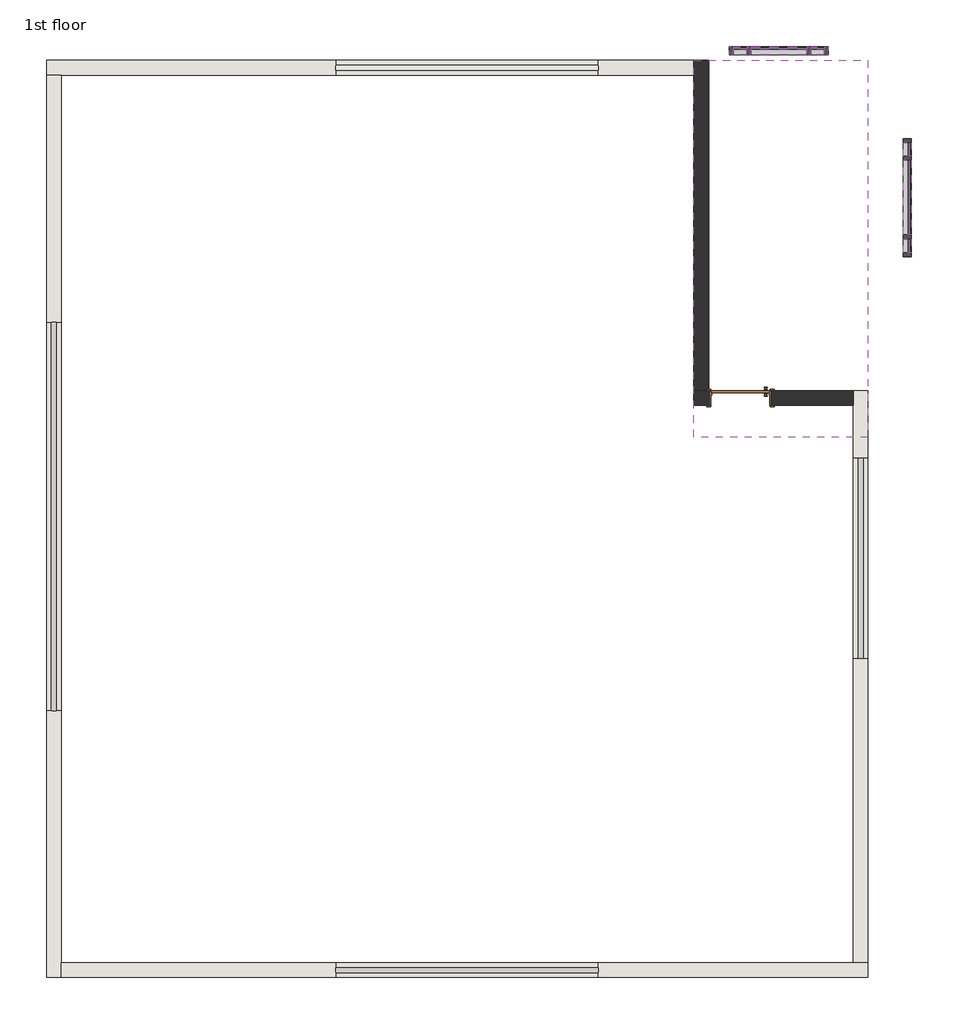
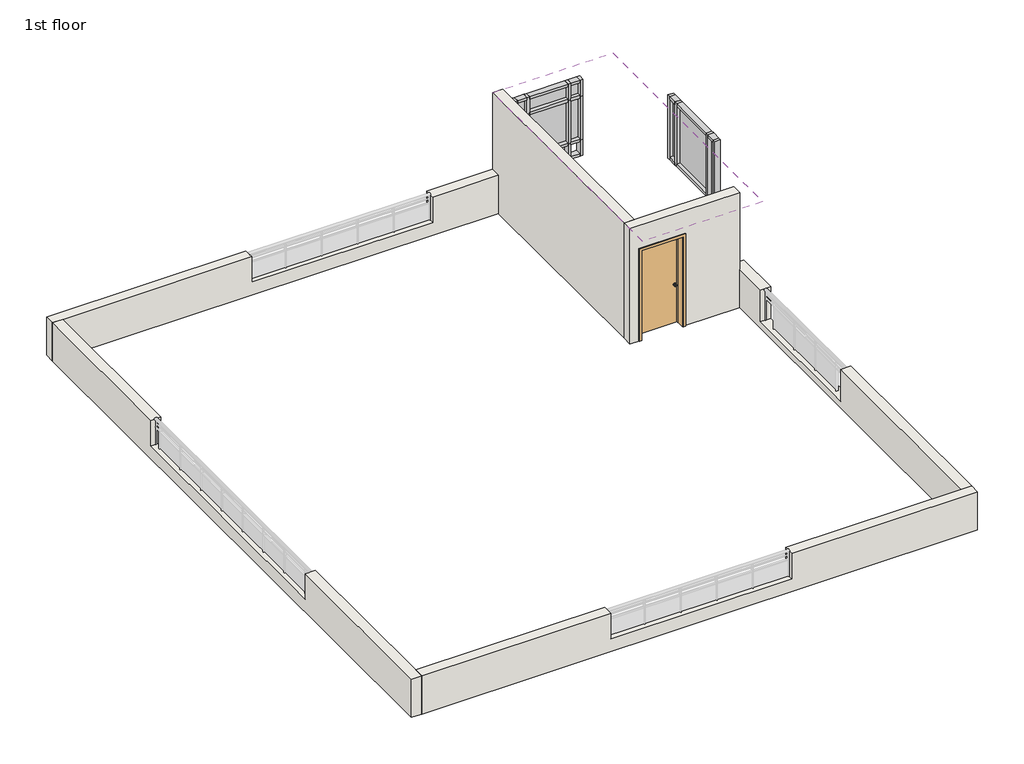
# One storey, part 1 of 2: 34 members, 9 plates, 6 walls, 1 door, 1 roof.
"""IFC4 building model written with IfcOpenShell, lengths in millimetres."""

from ifc_helpers import new_model, si_unit, frame, origin, place, context, project, spatial, polyline, outline, extrude, faceted_brep, transform, mapped, element, save
from components import door_b48525d3, member_420b45ef, member_90125dd4, member_1b4b4554, member_6b401d40, member_d98df40f, member_dfe75557, member_a5966c2a, member_b00ab025, member_467e6651, member_96c05505, member_8d8fe108, member_03a502dc, member_c5c38a7a, system_panel_glazed_475412f8, system_panel_glazed_19ddc366, system_panel_glazed_1899ac7a, system_panel_glazed_058753b2, system_panel_glazed_ee4e9f01, system_panel_glazed_f68cf4a2

model = new_model("IFC4")

# Units and contexts
model_context = context("Model", 3, world=origin())
ifc_project = project(units=[si_unit("LENGTHUNIT", "METRE", prefix="MILLI")], contexts=[model_context])

# Site, building, storey
site = spatial("IfcSite", under=ifc_project)
building = spatial("IfcBuilding", under=site)
storey = spatial("IfcBuildingStorey", under=building, Name="1st floor", Elevation=3200.4)

# Door
placement = place(None, origin())
door_shape = door_b48525d3(model_context)
element("IfcDoor", 1, ObjectType="Door-Interior-Single-Flush_Panel-Wood : 36\" x 84\"", at=placement, inside=storey, context=model_context, shape_type="MappedRepresentation", body=[
    mapped(door_shape, transform((-1718.0277598, 6738.9092801, 3200.4), x_axis=(-1.0, 0.0, 0.0), y_axis=(0.0, -1.0, 0.0), z_axis=(0.0, 0.0, 1.0))),
])

# Members
member_shape = member_420b45ef(model_context)
element("IfcMember", 2, ObjectType="Rectangular Mullion : 2.5\" x 5\" rectangular", at=placement, inside=storey, context=model_context, shape_type="MappedRepresentation", body=[
    mapped(member_shape, transform((872.7722402, 10703.2142801, 5486.4), x_axis=(0.0, 0.0, 1.0), y_axis=(1.0, 0.0, 0.0), z_axis=(0.0, 1.0, 0.0))),
])
element("IfcMember", 3, ObjectType="Rectangular Mullion : 2.5\" x 5\" rectangular", at=placement, inside=storey, context=model_context, shape_type="MappedRepresentation", body=[
    mapped(member_shape, transform((872.7722402, 9205.8842801, 5486.4), x_axis=(0.0, 0.0, 1.0), y_axis=(1.0, 0.0, 0.0), z_axis=(0.0, 1.0, 0.0))),
])
element("IfcMember", 4, ObjectType="Rectangular Mullion : 2.5\" x 5\" rectangular", at=placement, inside=storey, context=model_context, shape_type="MappedRepresentation", body=[
    mapped(member_shape, transform((-1828.7123825, 12133.2342801, 5481.32), x_axis=(0.0, 0.0, 1.0), y_axis=(0.0, 1.0, 0.0), z_axis=(-1.0, 0.0, 0.0))),
])
element("IfcMember", 5, ObjectType="Rectangular Mullion : 2.5\" x 5\" rectangular", at=placement, inside=storey, context=model_context, shape_type="MappedRepresentation", body=[
    mapped(member_shape, transform((-627.5183629, 12133.2342801, 5481.32), x_axis=(0.0, 0.0, 1.0), y_axis=(0.0, 1.0, 0.0), z_axis=(-1.0, 0.0, 0.0))),
])
member_2_shape = member_90125dd4(model_context)
element("IfcMember", 6, ObjectType="Rectangular Mullion : 2.5\" x 5\" rectangular", at=placement, inside=storey, context=model_context, shape_type="MappedRepresentation", body=[
    mapped(member_2_shape, transform((872.7722402, 8932.8342801, 5486.4), x_axis=(0.0, -1.0, 0.0), y_axis=(1.0, 0.0, 0.0), z_axis=(0.0, 0.0, 1.0))),
])
element("IfcMember", 7, ObjectType="Rectangular Mullion : 2.5\" x 5\" rectangular", at=placement, inside=storey, context=model_context, shape_type="MappedRepresentation", body=[
    mapped(member_shape, transform((872.7722402, 8996.3342801, 3976.7979445), x_axis=(0.0, 0.0, -1.0), y_axis=(1.0, 0.0, 0.0), z_axis=(0.0, -1.0, 0.0))),
])
element("IfcMember", 8, ObjectType="Rectangular Mullion : 2.5\" x 5\" rectangular", at=placement, inside=storey, context=model_context, shape_type="MappedRepresentation", body=[
    mapped(member_shape, transform((872.7722402, 10493.6642801, 3976.7979445), x_axis=(0.0, 0.0, -1.0), y_axis=(1.0, 0.0, 0.0), z_axis=(0.0, -1.0, 0.0))),
])
element("IfcMember", 9, ObjectType="Rectangular Mullion : 2.5\" x 5\" rectangular", at=placement, inside=storey, context=model_context, shape_type="MappedRepresentation", body=[
    mapped(member_shape, transform((-417.9683629, 12133.2342801, 3662.68), x_axis=(0.0, 0.0, -1.0), y_axis=(0.0, 1.0, 0.0), z_axis=(1.0, 0.0, 0.0))),
])
element("IfcMember", 10, ObjectType="Rectangular Mullion : 2.5\" x 5\" rectangular", at=placement, inside=storey, context=model_context, shape_type="MappedRepresentation", body=[
    mapped(member_shape, transform((-1619.1623825, 12133.2342801, 3662.68), x_axis=(0.0, 0.0, -1.0), y_axis=(0.0, 1.0, 0.0), z_axis=(1.0, 0.0, 0.0))),
])
element("IfcMember", 11, ObjectType="Rectangular Mullion : 2.5\" x 5\" rectangular", at=placement, inside=storey, context=model_context, shape_type="MappedRepresentation", body=[
    mapped(member_2_shape, transform((872.7722402, 10766.7142801, 3976.7979445), x_axis=(0.0, 1.0, 0.0), y_axis=(1.0, 0.0, 0.0), z_axis=(0.0, 0.0, -1.0))),
])
member_3_shape = member_1b4b4554(model_context)
element("IfcMember", 12, ObjectType="Rectangular Mullion : 2.5\" x 5\" rectangular", at=placement, inside=storey, context=model_context, shape_type="MappedRepresentation", body=[
    mapped(member_3_shape, transform((872.7722402, 9237.6342801, 5486.4), x_axis=(0.0, -1.0, 0.0), y_axis=(1.0, 0.0, 0.0), z_axis=(0.0, 0.0, 1.0))),
])
element("IfcMember", 13, ObjectType="Rectangular Mullion : 2.5\" x 5\" rectangular", at=placement, inside=storey, context=model_context, shape_type="MappedRepresentation", body=[
    mapped(member_3_shape, transform((872.7722402, 10461.9142801, 5486.4), x_axis=(0.0, -1.0, 0.0), y_axis=(1.0, 0.0, 0.0), z_axis=(0.0, 0.0, 1.0))),
])
member_4_shape = member_6b401d40(model_context)
element("IfcMember", 14, ObjectType="Rectangular Mullion : 2.5\" x 5\" rectangular", at=placement, inside=storey, context=model_context, shape_type="MappedRepresentation", body=[
    mapped(member_4_shape, transform((872.7722402, 10430.1642801, 5486.4), x_axis=(0.0, 0.0, 1.0), y_axis=(1.0, 0.0, 0.0), z_axis=(0.0, 1.0, 0.0))),
])
element("IfcMember", 15, ObjectType="Rectangular Mullion : 2.5\" x 5\" rectangular", at=placement, inside=storey, context=model_context, shape_type="MappedRepresentation", body=[
    mapped(member_4_shape, transform((872.7722402, 9269.3842801, 3976.7979445), x_axis=(0.0, 0.0, -1.0), y_axis=(1.0, 0.0, 0.0), z_axis=(0.0, -1.0, 0.0))),
])
member_5_shape = member_d98df40f(model_context)
element("IfcMember", 16, ObjectType="Rectangular Mullion : 2.5\" x 5\" rectangular", at=placement, inside=storey, context=model_context, shape_type="MappedRepresentation", body=[
    mapped(member_5_shape, transform((-354.4683629, 12133.2342801, 5481.32), x_axis=(1.0, 0.0, 0.0), y_axis=(0.0, 1.0, 0.0), z_axis=(0.0, 0.0, 1.0))),
])
member_6_shape = member_dfe75557(model_context)
element("IfcMember", 17, ObjectType="Rectangular Mullion : 2.5\" x 5\" rectangular", at=placement, inside=storey, context=model_context, shape_type="MappedRepresentation", body=[
    mapped(member_6_shape, transform((-1892.2123825, 12133.2342801, 3662.68), x_axis=(-1.0, 0.0, 0.0), y_axis=(0.0, 1.0, 0.0), z_axis=(0.0, 0.0, -1.0))),
])
member_7_shape = member_a5966c2a(model_context)
element("IfcMember", 18, ObjectType="Rectangular Mullion : 2.5\" x 5\" rectangular", at=placement, inside=storey, context=model_context, shape_type="MappedRepresentation", body=[
    mapped(member_7_shape, transform((-1828.7123825, 12133.2342801, 4043.68), x_axis=(0.0, 0.0, 1.0), y_axis=(0.0, 1.0, 0.0), z_axis=(-1.0, 0.0, 0.0))),
])
element("IfcMember", 19, ObjectType="Rectangular Mullion : 2.5\" x 5\" rectangular", at=placement, inside=storey, context=model_context, shape_type="MappedRepresentation", body=[
    mapped(member_7_shape, transform((-627.5183629, 12133.2342801, 4043.68), x_axis=(0.0, 0.0, 1.0), y_axis=(0.0, 1.0, 0.0), z_axis=(-1.0, 0.0, 0.0))),
])
element("IfcMember", 20, ObjectType="Rectangular Mullion : 2.5\" x 5\" rectangular", at=placement, inside=storey, context=model_context, shape_type="MappedRepresentation", body=[
    mapped(member_7_shape, transform((-1828.7123825, 12133.2342801, 5085.08), x_axis=(0.0, 0.0, 1.0), y_axis=(0.0, 1.0, 0.0), z_axis=(-1.0, 0.0, 0.0))),
])
element("IfcMember", 21, ObjectType="Rectangular Mullion : 2.5\" x 5\" rectangular", at=placement, inside=storey, context=model_context, shape_type="MappedRepresentation", body=[
    mapped(member_7_shape, transform((-627.5183629, 12133.2342801, 5085.08), x_axis=(0.0, 0.0, 1.0), y_axis=(0.0, 1.0, 0.0), z_axis=(-1.0, 0.0, 0.0))),
])
member_8_shape = member_b00ab025(model_context)
element("IfcMember", 22, ObjectType="Rectangular Mullion : 2.5\" x 5\" rectangular", at=placement, inside=storey, context=model_context, shape_type="MappedRepresentation", body=[
    mapped(member_8_shape, transform((-1555.6623825, 12133.2342801, 4043.68), x_axis=(0.0, 0.0, 1.0), y_axis=(0.0, 1.0, 0.0), z_axis=(-1.0, 0.0, 0.0))),
])
element("IfcMember", 23, ObjectType="Rectangular Mullion : 2.5\" x 5\" rectangular", at=placement, inside=storey, context=model_context, shape_type="MappedRepresentation", body=[
    mapped(member_8_shape, transform((-1555.6623825, 12133.2342801, 5085.08), x_axis=(0.0, 0.0, 1.0), y_axis=(0.0, 1.0, 0.0), z_axis=(-1.0, 0.0, 0.0))),
])
member_9_shape = member_467e6651(model_context)
element("IfcMember", 24, ObjectType="Rectangular Mullion : 2.5\" x 5\" rectangular", at=placement, inside=storey, context=model_context, shape_type="MappedRepresentation", body=[
    mapped(member_9_shape, transform((-659.2683629, 12133.2342801, 5481.32), x_axis=(1.0, 0.0, 0.0), y_axis=(0.0, 1.0, 0.0), z_axis=(0.0, 0.0, 1.0))),
])
element("IfcMember", 25, ObjectType="Rectangular Mullion : 2.5\" x 5\" rectangular", at=placement, inside=storey, context=model_context, shape_type="MappedRepresentation", body=[
    mapped(member_9_shape, transform((-1587.4123825, 12133.2342801, 5481.32), x_axis=(1.0, 0.0, 0.0), y_axis=(0.0, 1.0, 0.0), z_axis=(0.0, 0.0, 1.0))),
])
member_10_shape = member_96c05505(model_context)
element("IfcMember", 26, ObjectType="Rectangular Mullion : 2.5\" x 5\" rectangular", at=placement, inside=storey, context=model_context, shape_type="MappedRepresentation", body=[
    mapped(member_10_shape, transform((-1555.6623825, 12133.2342801, 5481.32), x_axis=(0.0, 0.0, 1.0), y_axis=(0.0, 1.0, 0.0), z_axis=(-1.0, 0.0, 0.0))),
])
element("IfcMember", 27, ObjectType="Rectangular Mullion : 2.5\" x 5\" rectangular", at=placement, inside=storey, context=model_context, shape_type="MappedRepresentation", body=[
    mapped(member_6_shape, transform((-354.4683629, 12133.2342801, 4043.68), x_axis=(1.0, 0.0, 0.0), y_axis=(0.0, 1.0, 0.0), z_axis=(0.0, 0.0, 1.0))),
])
member_11_shape = member_8d8fe108(model_context)
element("IfcMember", 28, ObjectType="Rectangular Mullion : 2.5\" x 5\" rectangular", at=placement, inside=storey, context=model_context, shape_type="MappedRepresentation", body=[
    mapped(member_11_shape, transform((-354.4683629, 12133.2342801, 5085.08), x_axis=(1.0, 0.0, 0.0), y_axis=(0.0, 1.0, 0.0), z_axis=(0.0, 0.0, 1.0))),
])
element("IfcMember", 29, ObjectType="Rectangular Mullion : 2.5\" x 5\" rectangular", at=placement, inside=storey, context=model_context, shape_type="MappedRepresentation", body=[
    mapped(member_10_shape, transform((-691.0183629, 12133.2342801, 3662.68), x_axis=(0.0, 0.0, -1.0), y_axis=(0.0, 1.0, 0.0), z_axis=(1.0, 0.0, 0.0))),
])
element("IfcMember", 30, ObjectType="Rectangular Mullion : 2.5\" x 5\" rectangular", at=placement, inside=storey, context=model_context, shape_type="MappedRepresentation", body=[
    mapped(member_11_shape, transform((-1892.2123825, 12133.2342801, 4043.68), x_axis=(-1.0, 0.0, 0.0), y_axis=(0.0, 1.0, 0.0), z_axis=(0.0, 0.0, -1.0))),
])
element("IfcMember", 31, ObjectType="Rectangular Mullion : 2.5\" x 5\" rectangular", at=placement, inside=storey, context=model_context, shape_type="MappedRepresentation", body=[
    mapped(member_5_shape, transform((-1892.2123825, 12133.2342801, 5085.08), x_axis=(-1.0, 0.0, 0.0), y_axis=(0.0, 1.0, 0.0), z_axis=(0.0, 0.0, -1.0))),
])
member_12_shape = member_03a502dc(model_context)
element("IfcMember", 32, ObjectType="Rectangular Mullion : 2.5\" x 5\" rectangular", at=placement, inside=storey, context=model_context, shape_type="MappedRepresentation", body=[
    mapped(member_12_shape, transform((-659.2683629, 12133.2342801, 4043.68), x_axis=(1.0, 0.0, 0.0), y_axis=(0.0, 1.0, 0.0), z_axis=(0.0, 0.0, 1.0))),
])
element("IfcMember", 33, ObjectType="Rectangular Mullion : 2.5\" x 5\" rectangular", at=placement, inside=storey, context=model_context, shape_type="MappedRepresentation", body=[
    mapped(member_12_shape, transform((-1587.4123825, 12133.2342801, 4043.68), x_axis=(1.0, 0.0, 0.0), y_axis=(0.0, 1.0, 0.0), z_axis=(0.0, 0.0, 1.0))),
])
member_13_shape = member_c5c38a7a(model_context)
element("IfcMember", 34, ObjectType="Rectangular Mullion : 2.5\" x 5\" rectangular", at=placement, inside=storey, context=model_context, shape_type="MappedRepresentation", body=[
    mapped(member_13_shape, transform((-659.2683629, 12133.2342801, 5085.08), x_axis=(1.0, 0.0, 0.0), y_axis=(0.0, 1.0, 0.0), z_axis=(0.0, 0.0, 1.0))),
])
element("IfcMember", 35, ObjectType="Rectangular Mullion : 2.5\" x 5\" rectangular", at=placement, inside=storey, context=model_context, shape_type="MappedRepresentation", body=[
    mapped(member_13_shape, transform((-1587.4123825, 12133.2342801, 5085.08), x_axis=(1.0, 0.0, 0.0), y_axis=(0.0, 1.0, 0.0), z_axis=(0.0, 0.0, 1.0))),
])

# Plates
system_panel_glazed_shape = system_panel_glazed_475412f8(model_context)
element("IfcPlate", 36, ObjectType="System Panel : Glazed", at=placement, inside=storey, context=model_context, shape_type="MappedRepresentation", body=[
    mapped(system_panel_glazed_shape, transform((872.7722402, 10598.4392801, 4040.2979445), x_axis=(0.0, -1.0, 0.0), y_axis=(1.0, 0.0, 0.0), z_axis=(0.0, 0.0, 1.0))),
])
element("IfcPlate", 37, ObjectType="System Panel : Glazed", at=placement, inside=storey, context=model_context, shape_type="MappedRepresentation", body=[
    mapped(system_panel_glazed_shape, transform((872.7722402, 9101.1092801, 4040.2979445), x_axis=(0.0, -1.0, 0.0), y_axis=(1.0, 0.0, 0.0), z_axis=(0.0, 0.0, 1.0))),
])
system_panel_glazed_2_shape = system_panel_glazed_19ddc366(model_context)
element("IfcPlate", 38, ObjectType="System Panel : Glazed", at=placement, inside=storey, context=model_context, shape_type="MappedRepresentation", body=[
    mapped(system_panel_glazed_2_shape, transform((872.7722402, 9849.7742801, 4040.2979445), x_axis=(0.0, -1.0, 0.0), y_axis=(1.0, 0.0, 0.0), z_axis=(0.0, 0.0, 1.0))),
])
system_panel_glazed_3_shape = system_panel_glazed_1899ac7a(model_context)
element("IfcPlate", 39, ObjectType="System Panel : Glazed", at=placement, inside=storey, context=model_context, shape_type="MappedRepresentation", body=[
    mapped(system_panel_glazed_3_shape, transform((-1723.9373825, 12133.2342801, 4075.43), x_axis=(1.0, 0.0, 0.0), y_axis=(0.0, 1.0, 0.0), z_axis=(0.0, 0.0, 1.0))),
])
element("IfcPlate", 40, ObjectType="System Panel : Glazed", at=placement, inside=storey, context=model_context, shape_type="MappedRepresentation", body=[
    mapped(system_panel_glazed_3_shape, transform((-522.7433629, 12133.2342801, 4075.43), x_axis=(1.0, 0.0, 0.0), y_axis=(0.0, 1.0, 0.0), z_axis=(0.0, 0.0, 1.0))),
])
system_panel_glazed_4_shape = system_panel_glazed_058753b2(model_context)
element("IfcPlate", 41, ObjectType="System Panel : Glazed", at=placement, inside=storey, context=model_context, shape_type="MappedRepresentation", body=[
    mapped(system_panel_glazed_4_shape, transform((-1723.9373825, 12133.2342801, 5116.83), x_axis=(1.0, 0.0, 0.0), y_axis=(0.0, 1.0, 0.0), z_axis=(0.0, 0.0, 1.0))),
])
element("IfcPlate", 42, ObjectType="System Panel : Glazed", at=placement, inside=storey, context=model_context, shape_type="MappedRepresentation", body=[
    mapped(system_panel_glazed_4_shape, transform((-522.7433629, 12133.2342801, 5116.83), x_axis=(1.0, 0.0, 0.0), y_axis=(0.0, 1.0, 0.0), z_axis=(0.0, 0.0, 1.0))),
])
system_panel_glazed_5_shape = system_panel_glazed_ee4e9f01(model_context)
element("IfcPlate", 43, ObjectType="System Panel : Glazed", at=placement, inside=storey, context=model_context, shape_type="MappedRepresentation", body=[
    mapped(system_panel_glazed_5_shape, transform((-1123.3403727, 12133.2342801, 4075.43), x_axis=(1.0, 0.0, 0.0), y_axis=(0.0, 1.0, 0.0), z_axis=(0.0, 0.0, 1.0))),
])
system_panel_glazed_6_shape = system_panel_glazed_f68cf4a2(model_context)
element("IfcPlate", 44, ObjectType="System Panel : Glazed", at=placement, inside=storey, context=model_context, shape_type="MappedRepresentation", body=[
    mapped(system_panel_glazed_6_shape, transform((-1123.3403727, 12133.2342801, 5116.83), x_axis=(1.0, 0.0, 0.0), y_axis=(0.0, 1.0, 0.0), z_axis=(0.0, 0.0, 1.0))),
])

# Roof
element("IfcRoof", 45, ObjectType="Generic - 6\"", at=placement, inside=storey, context=model_context, shape_type="SweptSolid", body=[
    extrude(outline(polyline([(-2441.9277598, 11980.8342801), (263.1722402, 11980.8342801), (263.1722402, 6126.1342801), (-2441.9277598, 6126.1342801), (-2441.9277598, 11980.8342801)])), frame((0.0, 0.0, 5943.6), z_axis=(0.0, 0.0, 1.0), x_axis=(1.0, 0.0, 0.0)), (0.0, 0.0, 1.0), 152.4),
])

# Walls
element("IfcWall", 46, ObjectType="Generic - 9\"", at=placement, inside=storey, context=model_context, shape_type="Brep", body=[
    faceted_brep([(-12500.3277598, 11752.2342801, 3200.4), (-12271.7277598, 11752.2342801, 3200.4), (-2441.9277598, 11752.2342801, 3200.4), (-2441.9277598, 11752.2342801, 4114.8), (-3926.753987, 11752.2342801, 4114.8), (-3926.753987, 11752.2342801, 3505.2), (-8005.6015325, 11752.2342801, 3505.2), (-8005.6015325, 11752.2342801, 4114.8), (-12271.7277598, 11752.2342801, 4114.8), (-12500.3277598, 11752.2342801, 4114.8), (-12500.3277598, 11980.8342801, 3200.4), (-12500.3277598, 11980.8342801, 4114.8), (-8005.6015325, 11980.8342801, 4114.8), (-8005.6015325, 11980.8342801, 3505.2), (-3926.753987, 11980.8342801, 3505.2), (-3926.753987, 11980.8342801, 4114.8), (-2441.9277598, 11980.8342801, 4114.8), (-2441.9277598, 11980.8342801, 3200.4)], [[[0, 1, 2, 3, 4, 5, 6, 7, 8, 9]], [[10, 11, 12, 13, 14, 15, 16, 17]], [[0, 9, 11, 10]], [[3, 2, 17, 16]], [[2, 1, 0, 10, 17]], [[4, 3, 16, 15]], [[5, 4, 15, 14]], [[6, 5, 14, 13]], [[7, 6, 13, 12]], [[9, 8, 7, 12, 11]]]),
])
element("IfcWall", 47, ObjectType="Generic - 9\"", at=placement, inside=storey, context=model_context, shape_type="Brep", body=[
    faceted_brep([(-12500.3277598, 11752.2342801, 3200.4), (-12500.3277598, -2268.5657199, 3200.4), (-12500.3277598, -2268.5657199, 4114.8), (-12500.3277598, 1879.1217625, 4114.8), (-12500.3277598, 1879.1217625, 3505.2), (-12500.3277598, 7909.3467978, 3505.2), (-12500.3277598, 7909.3467978, 4114.8), (-12500.3277598, 11752.2342801, 4114.8), (-12271.7277598, 11752.2342801, 3200.4), (-12271.7277598, 11752.2342801, 4114.8), (-12271.7277598, 7909.3467978, 4114.8), (-12271.7277598, 7909.3467978, 3505.2), (-12271.7277598, 1879.1217625, 3505.2), (-12271.7277598, 1879.1217625, 4114.8), (-12271.7277598, -2039.9657199, 4114.8), (-12271.7277598, -2268.5657199, 4114.8), (-12271.7277598, -2268.5657199, 3200.4), (-12271.7277598, -2039.9657199, 3200.4)], [[[0, 1, 2, 3, 4, 5, 6, 7]], [[8, 9, 10, 11, 12, 13, 14, 15, 16, 17]], [[0, 7, 9, 8]], [[2, 1, 16, 15]], [[1, 0, 8, 17, 16]], [[3, 2, 15, 14, 13]], [[4, 3, 13, 12]], [[5, 4, 12, 11]], [[6, 5, 11, 10]], [[7, 6, 10, 9]]]),
])
element("IfcWall", 48, ObjectType="Generic - 9\"", at=placement, inside=storey, context=model_context, shape_type="Brep", body=[
    faceted_brep([(-12271.7277598, -2268.5657199, 3200.4), (263.1722402, -2268.5657199, 3200.4), (263.1722402, -2268.5657199, 4114.8), (-3926.753987, -2268.5657199, 4114.8), (-3926.753987, -2268.5657199, 3505.2), (-8005.6015325, -2268.5657199, 3505.2), (-8005.6015325, -2268.5657199, 4114.8), (-12271.7277598, -2268.5657199, 4114.8), (-12271.7277598, -2039.9657199, 3200.4), (-12271.7277598, -2039.9657199, 4114.8), (-8005.6015325, -2039.9657199, 4114.8), (-8005.6015325, -2039.9657199, 3505.2), (-3926.753987, -2039.9657199, 3505.2), (-3926.753987, -2039.9657199, 4114.8), (34.5722402, -2039.9657199, 4114.8), (263.1722402, -2039.9657199, 4114.8), (263.1722402, -2039.9657199, 3200.4), (34.5722402, -2039.9657199, 3200.4)], [[[0, 1, 2, 3, 4, 5, 6, 7]], [[8, 9, 10, 11, 12, 13, 14, 15, 16, 17]], [[0, 7, 9, 8]], [[2, 1, 16, 15]], [[1, 0, 8, 17, 16]], [[3, 2, 15, 14, 13]], [[4, 3, 13, 12]], [[5, 4, 12, 11]], [[6, 5, 11, 10]], [[7, 6, 10, 9]]]),
])
element("IfcWall", 49, ObjectType="Generic - 9\"", at=placement, inside=storey, context=model_context, shape_type="Brep", body=[
    faceted_brep([(263.1722402, -2039.9657199, 3200.4), (263.1722402, 6850.0342801, 3200.4), (263.1722402, 6850.0342801, 4114.8), (263.1722402, 5808.6342801, 4114.8), (263.1722402, 5808.6342801, 3352.8), (263.1722402, 2680.2485536, 3352.8), (263.1722402, 2680.2485536, 4114.8), (263.1722402, -2039.9657199, 4114.8), (34.5722402, -2039.9657199, 3200.4), (34.5722402, -2039.9657199, 4114.8), (34.5722402, 2680.2485536, 4114.8), (34.5722402, 2680.2485536, 3352.8), (34.5722402, 5808.6342801, 3352.8), (34.5722402, 5808.6342801, 4114.8), (34.5722402, 6850.0342801, 4114.8), (34.5722402, 6850.0342801, 3200.4), (34.5722402, 6621.4342801, 3200.4)], [[[0, 1, 2, 3, 4, 5, 6, 7]], [[8, 9, 10, 11, 12, 13, 14, 15, 16]], [[0, 7, 9, 8]], [[2, 1, 15, 14]], [[1, 0, 8, 16, 15]], [[7, 6, 10, 9]], [[3, 2, 14, 13]], [[4, 3, 13, 12]], [[5, 4, 12, 11]], [[6, 5, 11, 10]]]),
])
element("IfcWall", 50, ObjectType="Generic - 9\"", at=placement, inside=storey, context=model_context, shape_type="Brep", body=[
    faceted_brep([(-2441.9277598, 6850.0342801, 5943.6), (-2213.3277598, 6850.0342801, 5943.6), (34.5722402, 6850.0342801, 5943.6), (34.5722402, 6850.0342801, 4114.8), (34.5722402, 6850.0342801, 3200.4), (-1235.4277598, 6850.0342801, 3200.4), (-1235.4277598, 6850.0342801, 5359.4), (-2200.6277598, 6850.0342801, 5359.4), (-2200.6277598, 6850.0342801, 3200.4), (-2213.3277598, 6850.0342801, 3200.4), (-2441.9277598, 6850.0342801, 3200.4), (34.5722402, 6621.4342801, 5943.6), (-2441.9277598, 6621.4342801, 5943.6), (-2441.9277598, 6621.4342801, 3200.4), (-2200.6277598, 6621.4342801, 3200.4), (-2200.6277598, 6621.4342801, 5359.4), (-1235.4277598, 6621.4342801, 5359.4), (-1235.4277598, 6621.4342801, 3200.4), (34.5722402, 6621.4342801, 3200.4)], [[[0, 1, 2, 3, 4, 5, 6, 7, 8, 9, 10]], [[11, 12, 13, 14, 15, 16, 17, 18]], [[4, 18, 17, 5]], [[13, 10, 9, 8, 14]], [[2, 1, 0, 12, 11]], [[0, 10, 13, 12]], [[7, 15, 14, 8]], [[15, 7, 6, 16]], [[16, 6, 5, 17]], [[18, 4, 3, 2, 11]]]),
])
element("IfcWall", 51, ObjectType="Generic - 9\"", at=placement, inside=storey, context=model_context, shape_type="Brep", body=[
    faceted_brep([(-2213.3277598, 6850.0342801, 3200.4), (-2213.3277598, 11980.8342801, 3200.4), (-2213.3277598, 11980.8342801, 5943.6), (-2213.3277598, 6850.0342801, 5943.6), (-2441.9277598, 6850.0342801, 3200.4), (-2441.9277598, 6850.0342801, 5943.6), (-2441.9277598, 11980.8342801, 5943.6), (-2441.9277598, 11980.8342801, 4114.8), (-2441.9277598, 11980.8342801, 3200.4), (-2441.9277598, 11752.2342801, 3200.4)], [[[0, 1, 2, 3]], [[4, 5, 6, 7, 8, 9]], [[1, 0, 4, 9, 8]], [[3, 2, 6, 5]], [[2, 1, 8, 7, 6]], [[0, 3, 5, 4]]]),
])

save(model, "model.ifc")

# Revit data of these elements
# Type "Door-Interior-Single-Flush_Panel-Wood : 36\" x 84\""
#   Type Mark = "12"
#   Analytic Construction = "Wooden"
#   Thickness = 0' - 1 3/8"
#   Thermal Resistance (R) = 2.5876 (h·ft²·°F)/BTU
#   Swing Angle [instance default] = 90.00°
#   Rough Width = 3' - 2"
#   Rough Height = 7' - 1"
#   Height = 7' - 0"
#   Width = 3' - 0"
#   Heat Transfer Coefficient (U) = 0.3865 BTU/(h·ft²·°F)
#   Trim Material = Cherry
#   Panel Material = Cherry
#   Frame Material = Cherry
#   Door Handle Material = Aluminum
#   Visual Light Transmittance = 0
#   Solar Heat Gain Coefficient = 0
#   Wall Closure = (empty or 0)
#   Function = (empty or 0)
# Type "Rectangular Mullion : 2.5\" x 5\" rectangular"
#   built-in parameter 1007304 = 0.416667 (stored number, unit not read)
#   built-in parameter 1007301 = 0.104167 (stored number, unit not read)
#   built-in parameter 1007300 = 0.104167 (stored number, unit not read)
# Type "System Panel : Glazed"
#   Construction Type Id = "GSP4R"
#   Analytic Construction = "1/8 in Pilkington single glazing"
#   Visual Light Transmittance = 0.9
#   Solar Heat Gain Coefficient = 0.86
#   Heat Transfer Coefficient (U) = 1.18115 BTU/(h·ft²·°F)
#   Define Thermal Properties by = 1
# Type "Generic - 6\""
#   Layers, outside or top first: 0' - 6" "Concrete, Precast" (function 1)
# Type "Generic - 9\""
#   Layers, outside or top first: 0' - 0 1/2" no material (function 4); 0' - 8" "Brick, Common" (function 1); 0' - 0 1/2" no material (function 5)
# Element 1 (IfcDoor, "Door-Interior-Single-Flush_Panel-Wood : 36\" x 84\"")
#   Swing Angle = 90.00°
#   Phase Created = New Construction
#   Materials on its faces: "Cherry", "Aluminum"
# Elements 2, 3, 4, 5, 6, 7, 8, 9, 10, 11, 12, 13, 14, 15, 16, 17, 18, 19, 20, 21, 22, 23, 24, 25, 26, 27, 28, 29, 30, 31, 32, 33, 34, 35 (IfcMember, "Rectangular Mullion : 2.5\" x 5\" rectangular")
#   Phase Created = New Construction
#   Materials on its faces: "Aluminum"
# Elements 36, 37, 38, 39, 40, 41, 42, 43, 44 (IfcPlate, "System Panel : Glazed")
#   Phase Created = New Construction
#   Materials on its faces: "Glass"
# Element 45 (IfcRoof, "Generic - 6\"")
#   built-in parameter 1001705 = 20 (stored number, unit not read)
#   built-in parameter 1001701 = 9 (stored number, unit not read)
#   built-in parameter 1001710 = 33615
#   Phase Created = New Construction
#   Materials on its faces: "Concrete, Precast"
# Elements 46, 47, 48, 49 (IfcWall, "Generic - 9\"")
#   Top Offset = -0' - 6"
#   Base Offset = 0' - 0"
#   Unconnected Height = 3' - 0"
#   wall height = 3' - 0"
#   Phase Created = New Construction
#   Base Constraint = 1st floor
#   Materials on its faces: "Default Wall"
# Elements 50, 51 (IfcWall, "Generic - 9\"")
#   Top Offset = -0' - 6"
#   Base Offset = 0' - 0"
#   Unconnected Height = 9' - 0"
#   wall height = 9' - 0"
#   Phase Created = New Construction
#   Base Constraint = 1st floor
#   Materials on its faces: "Default Wall"
# Materials
#   "Cherry": class "Wood", colour RGB 226 177 128, transparency 0, Description = "Prunus Serotina", Cost = 0
#   "Aluminum": class "Metal", colour RGB 247 247 247, transparency 0, Description = "Aluminum 6061", Cost = 0
#   "Concrete, Precast": class "Concrete", colour RGB 130 132 119, transparency 0, Description = "Precast concrete", Cost = 0
#   "Brick, Common": class "Masonry", colour RGB 85 47 55, transparency 0, Description = "Common brick", Cost = 0
#   "Glass": class "Glass", colour RGB 0 128 192, transparency 0.75, Description = "Soda Lime Glass", Cost = 0
#   "Default Wall": colour RGB 128 128 128, transparency 0, Cost = 0
